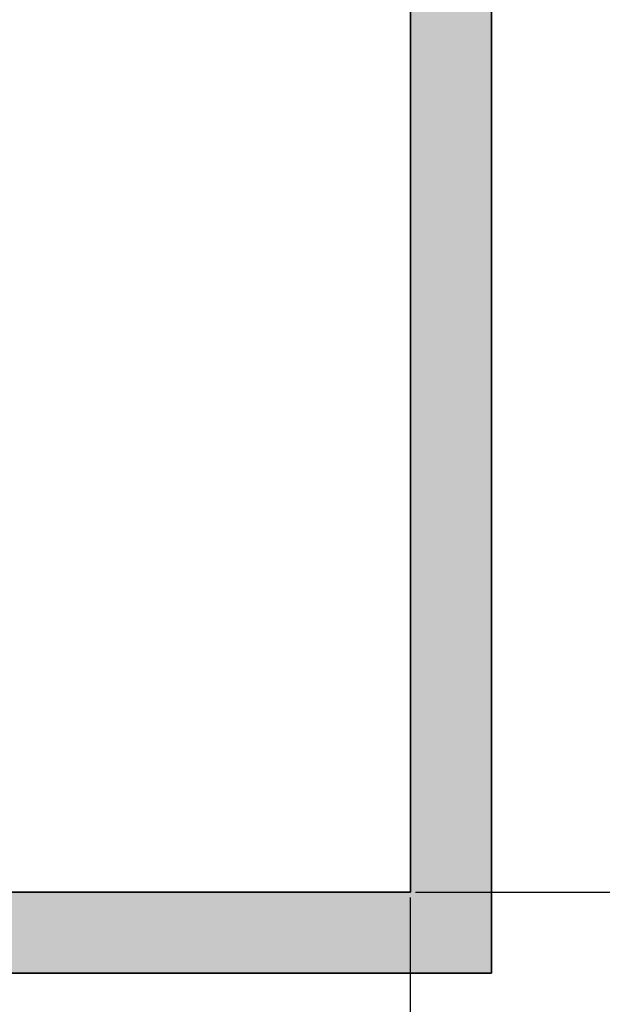
# Model space of a CAD drawing. Units: millimetres. Extents: x -22994 to 29398, y -19990 to 20176.
# Tile 36 of 135: x 183.3 to 190.48, y 29.61 to 41.76. Entities that reach past the tile are written whole.
import ezdxf
from ezdxf import colors
from ezdxf.entities.mleader import LeaderData, LeaderLine
from ezdxf.math import Vec2, Vec3

# ---------------------------------------------------------------- set-up
doc = ezdxf.new("R2010")
doc.units = ezdxf.units.MM
doc.header["$MEASUREMENT"] = 0
for name, color, linetype, lineweight in [('M-ANNO-TEXT', 7, 'Continuous', 25), ('M-DIMS', 2, 'Continuous', 18), ('M-EQPM-PATT', 7, 'Continuous', 18), ('M-PIPE', 7, 'Continuous', 35)]:
    doc.layers.add(name, color=color, linetype=linetype, lineweight=lineweight)
doc.styles.get("Standard").update_dxf_attribs({"font": 'arial.ttf'})
doc.dimstyles.get("Standard").update_dxf_attribs({"dimtxt": 0.18, "dimasz": 10000, "dimexe": 0.18, "dimexo": 0.0625, "dimgap": 0.09, "dimtad": 0, "dimtih": 1, "dimtoh": 1, "dimdec": 0, "dimzin": 0, "dimdsep": 46, "dimtxsty": 'Standard', "dimcen": 0.09, "dimadec": 0, "dimazin": 0, "dimtfac": 1, "dimtdec": 0, "dimtofl": 0, "dimtmove": 0, "dimatfit": 3, "dimfxl": 1, "dimtolj": 1, "dimtzin": 0, "dimlwd": 30, "dimarcsym": 0})

# ---------------------------------------------------------------- blocks, each defined once
blk = doc.blocks.new('*D2')
at = {"layer": 'Defpoints', "color": 0, "transparency": 16777216}
for p in [(6.677, 10.271), (290.852, 10.271), (290.852, -5.079)]:
    blk.add_point(p, dxfattribs=at)
at = {"layer": 'M-DIMS', "color": 0, "lineweight": -2, "transparency": 16777216}
for p, q in [((6.677, 10.209), (6.677, -5.259)), ((290.852, 10.209), (290.852, -5.259))]:
    blk.add_line(p, q, dxfattribs=at)
at = {"layer": 'M-DIMS', "color": 0, "lineweight": 30, "transparency": 16777216}
for p, q in [((-9993.323, -5.079), (-19993.323, -5.079)), ((10290.852, -5.079), (20290.852, -5.079))]:
    blk.add_line(p, q, dxfattribs=at)
at = {"layer": 'M-DIMS', "color": 0, "transparency": 16777216}
for points in [[(-9993.323, 1661.588), (-9993.323, -1671.745), (6.677, -5.079)], [(10290.852, 1661.588), (10290.852, -1671.745), (290.852, -5.079)]]:
    blk.add_solid(points, dxfattribs=at)
at = {"layer": 'M-DIMS', "color": 0, "transparency": 16777216, "insert": (148.765, -5.079), "char_height": 0.18, "attachment_point": 5}
blk.add_mtext('\\A1;284.2', dxfattribs=at)
blk = doc.blocks.new('*D3')
at = {"layer": 'Defpoints', "color": 0, "transparency": 16777216}
for p in [(110.265, 204.165), (110.265, 176.366), (95.833, 127.967)]:
    blk.add_point(p, dxfattribs=at)
at = {"layer": 'M-DIMS', "color": 0, "lineweight": -2, "transparency": 16777216}
for p, q in [((95.833, 128.03), (95.833, 204.345)), ((110.265, 176.429), (110.265, 204.345))]:
    blk.add_line(p, q, dxfattribs=at)
at = {"layer": 'M-DIMS', "color": 0, "lineweight": 30, "transparency": 16777216}
for p, q in [((-9904.167, 204.165), (-19904.167, 204.165)), ((10110.265, 204.165), (20110.265, 204.165))]:
    blk.add_line(p, q, dxfattribs=at)
at = {"layer": 'M-DIMS', "color": 0, "transparency": 16777216}
for points in [[(-9904.167, 1870.832), (-9904.167, -1462.501), (95.833, 204.165)], [(10110.265, 1870.832), (10110.265, -1462.501), (110.265, 204.165)]]:
    blk.add_solid(points, dxfattribs=at)
at = {"layer": 'M-DIMS', "color": 0, "transparency": 16777216, "insert": (103.049, 204.165), "char_height": 0.18, "attachment_point": 5}
blk.add_mtext('\\A1;14.432', dxfattribs=at)
blk = doc.blocks.new('*D4')
at = {"layer": 'Defpoints', "color": 0, "transparency": 16777216}
for p in [(116.265, 204.165), (110.265, 176.366), (116.265, 176.366)]:
    blk.add_point(p, dxfattribs=at)
at = {"layer": 'M-DIMS', "color": 0, "lineweight": -2, "transparency": 16777216}
for p, q in [((110.265, 176.429), (110.265, 204.345)), ((116.265, 176.429), (116.265, 204.345))]:
    blk.add_line(p, q, dxfattribs=at)
at = {"layer": 'M-DIMS', "color": 0, "lineweight": 30, "transparency": 16777216}
for p, q in [((-9889.735, 204.165), (-19889.735, 204.165)), ((10116.265, 204.165), (20116.265, 204.165))]:
    blk.add_line(p, q, dxfattribs=at)
at = {"layer": 'M-DIMS', "color": 0, "transparency": 16777216}
for points in [[(-9889.735, 1870.832), (-9889.735, -1462.501), (110.265, 204.165)], [(10116.265, 1870.832), (10116.265, -1462.501), (116.265, 204.165)]]:
    blk.add_solid(points, dxfattribs=at)
at = {"layer": 'M-DIMS', "color": 0, "transparency": 16777216, "insert": (113.265, 204.165), "char_height": 0.18, "attachment_point": 5}
blk.add_mtext('\\A1;6', dxfattribs=at)
blk = doc.blocks.new('*D5')
at = {"layer": 'Defpoints', "color": 0, "transparency": 16777216}
for p in [(181.265, 204.165), (116.265, 176.366), (181.265, 176.366)]:
    blk.add_point(p, dxfattribs=at)
at = {"layer": 'M-DIMS', "color": 0, "lineweight": -2, "transparency": 16777216}
for p, q in [((116.265, 176.429), (116.265, 204.345)), ((181.265, 176.429), (181.265, 204.345))]:
    blk.add_line(p, q, dxfattribs=at)
at = {"layer": 'M-DIMS', "color": 0, "lineweight": 30, "transparency": 16777216}
for p, q in [((-9883.735, 204.165), (-19883.735, 204.165)), ((10181.265, 204.165), (20181.265, 204.165))]:
    blk.add_line(p, q, dxfattribs=at)
at = {"layer": 'M-DIMS', "color": 0, "transparency": 16777216}
for points in [[(-9883.735, 1870.832), (-9883.735, -1462.501), (116.265, 204.165)], [(10181.265, 1870.832), (10181.265, -1462.501), (181.265, 204.165)]]:
    blk.add_solid(points, dxfattribs=at)
at = {"layer": 'M-DIMS', "color": 0, "transparency": 16777216, "insert": (148.765, 204.165), "char_height": 0.18, "attachment_point": 5}
blk.add_mtext('\\A1;65', dxfattribs=at)
blk = doc.blocks.new('*D6')
at = {"layer": 'Defpoints', "color": 0, "transparency": 16777216}
for p in [(187.265, 204.165), (181.265, 176.366), (187.265, 176.366)]:
    blk.add_point(p, dxfattribs=at)
at = {"layer": 'M-DIMS', "color": 0, "lineweight": -2, "transparency": 16777216}
for p, q in [((181.265, 176.429), (181.265, 204.345)), ((187.265, 176.429), (187.265, 204.345))]:
    blk.add_line(p, q, dxfattribs=at)
at = {"layer": 'M-DIMS', "color": 0, "lineweight": 30, "transparency": 16777216}
for p, q in [((-9818.735, 204.165), (-19818.735, 204.165)), ((10187.265, 204.165), (20187.265, 204.165))]:
    blk.add_line(p, q, dxfattribs=at)
at = {"layer": 'M-DIMS', "color": 0, "transparency": 16777216}
for points in [[(-9818.735, 1870.832), (-9818.735, -1462.501), (181.265, 204.165)], [(10187.265, 1870.832), (10187.265, -1462.501), (187.265, 204.165)]]:
    blk.add_solid(points, dxfattribs=at)
at = {"layer": 'M-DIMS', "color": 0, "transparency": 16777216, "insert": (184.265, 204.165), "char_height": 0.18, "attachment_point": 5}
blk.add_mtext('\\A1;6', dxfattribs=at)
blk = doc.blocks.new('*D7')
at = {"layer": 'Defpoints', "color": 0, "transparency": 16777216}
for p in [(201.697, 204.165), (187.265, 176.366), (201.697, 127.967)]:
    blk.add_point(p, dxfattribs=at)
at = {"layer": 'M-DIMS', "color": 0, "lineweight": -2, "transparency": 16777216}
for p, q in [((187.265, 176.429), (187.265, 204.345)), ((201.697, 128.03), (201.697, 204.345))]:
    blk.add_line(p, q, dxfattribs=at)
at = {"layer": 'M-DIMS', "color": 0, "lineweight": 30, "transparency": 16777216}
for p, q in [((-9812.735, 204.165), (-19812.735, 204.165)), ((10201.697, 204.165), (20201.697, 204.165))]:
    blk.add_line(p, q, dxfattribs=at)
at = {"layer": 'M-DIMS', "color": 0, "transparency": 16777216}
for points in [[(-9812.735, 1870.832), (-9812.735, -1462.501), (187.265, 204.165)], [(10201.697, 1870.832), (10201.697, -1462.501), (201.697, 204.165)]]:
    blk.add_solid(points, dxfattribs=at)
at = {"layer": 'M-DIMS', "color": 0, "transparency": 16777216, "insert": (194.481, 204.165), "char_height": 0.18, "attachment_point": 5}
blk.add_mtext('\\A1;14.432', dxfattribs=at)
blk = doc.blocks.new('*D8')
at = {"layer": 'Defpoints', "color": 0, "transparency": 16777216}
for p in [(227.648, 204.165), (227.648, 146.73), (201.697, 127.967)]:
    blk.add_point(p, dxfattribs=at)
at = {"layer": 'M-DIMS', "color": 0, "lineweight": -2, "transparency": 16777216}
for p, q in [((201.697, 128.03), (201.697, 204.345)), ((227.648, 146.792), (227.648, 204.345))]:
    blk.add_line(p, q, dxfattribs=at)
at = {"layer": 'M-DIMS', "color": 0, "lineweight": 30, "transparency": 16777216}
for p, q in [((-9798.303, 204.165), (-19798.303, 204.165)), ((10227.648, 204.165), (20227.648, 204.165))]:
    blk.add_line(p, q, dxfattribs=at)
at = {"layer": 'M-DIMS', "color": 0, "transparency": 16777216}
for points in [[(-9798.303, 1870.832), (-9798.303, -1462.501), (201.697, 204.165)], [(10227.648, 1870.832), (10227.648, -1462.501), (227.648, 204.165)]]:
    blk.add_solid(points, dxfattribs=at)
at = {"layer": 'M-DIMS', "color": 0, "transparency": 16777216, "insert": (214.673, 204.165), "char_height": 0.18, "attachment_point": 5}
blk.add_mtext('\\A1;25.95', dxfattribs=at)
blk = doc.blocks.new('*D9')
at = {"layer": 'Defpoints', "color": 0, "transparency": 16777216}
for p in [(187.265, 176.366), (306.202, 176.366), (290.852, 10.271)]:
    blk.add_point(p, dxfattribs=at)
at = {"layer": 'M-DIMS', "color": 0, "lineweight": 30, "transparency": 16777216}
for p, q in [((306.202, 10176.366), (306.202, 20176.366)), ((306.202, -9989.729), (306.202, -19989.729))]:
    blk.add_line(p, q, dxfattribs=at)
at = {"layer": 'M-DIMS', "color": 0, "lineweight": -2, "transparency": 16777216}
for p, q in [((187.327, 176.366), (306.382, 176.366)), ((290.915, 10.271), (306.382, 10.271))]:
    blk.add_line(p, q, dxfattribs=at)
at = {"layer": 'M-DIMS', "color": 0, "transparency": 16777216}
for points in [[(-1360.465, 10176.366), (1972.869, 10176.366), (306.202, 176.366)], [(-1360.465, -9989.729), (1972.869, -9989.729), (306.202, 10.271)]]:
    blk.add_solid(points, dxfattribs=at)
at = {"layer": 'M-DIMS', "color": 0, "transparency": 16777216, "insert": (306.202, 93.319), "char_height": 0.18, "attachment_point": 5}
blk.add_mtext('\\A1;166.1', dxfattribs=at)
blk = doc.blocks.new('*D10')
at = {"layer": 'Defpoints', "color": 0, "transparency": 16777216}
for p in [(125.65, 136.071), (133.346, 136.071), (133.346, -5.079)]:
    blk.add_point(p, dxfattribs=at)
at = {"layer": 'M-DIMS', "color": 0, "lineweight": -2, "transparency": 16777216}
for p, q in [((125.65, 136.009), (125.65, -5.259)), ((133.346, 136.009), (133.346, -5.259))]:
    blk.add_line(p, q, dxfattribs=at)
at = {"layer": 'M-DIMS', "color": 0, "lineweight": 30, "transparency": 16777216}
for p, q in [((-9874.35, -5.079), (-19874.35, -5.079)), ((10133.346, -5.079), (20133.346, -5.079))]:
    blk.add_line(p, q, dxfattribs=at)
at = {"layer": 'M-DIMS', "color": 0, "transparency": 16777216}
for points in [[(-9874.35, 1661.588), (-9874.35, -1671.745), (125.65, -5.079)], [(10133.346, 1661.588), (10133.346, -1671.745), (133.346, -5.079)]]:
    blk.add_solid(points, dxfattribs=at)
at = {"layer": 'M-DIMS', "color": 0, "transparency": 16777216, "insert": (129.498, -5.079), "char_height": 0.18, "attachment_point": 5}
blk.add_mtext('\\A1;7.696', dxfattribs=at)
blk = doc.blocks.new('*D11')
at = {"layer": 'Defpoints', "color": 0, "transparency": 16777216}
for p in [(133.346, 136.071), (135.65, 136.071), (135.65, -5.079)]:
    blk.add_point(p, dxfattribs=at)
at = {"layer": 'M-DIMS', "color": 0, "lineweight": -2, "transparency": 16777216}
for p, q in [((133.346, 136.009), (133.346, -5.259)), ((135.65, 136.009), (135.65, -5.259))]:
    blk.add_line(p, q, dxfattribs=at)
at = {"layer": 'M-DIMS', "color": 0, "lineweight": 30, "transparency": 16777216}
for p, q in [((-9866.654, -5.079), (-19866.654, -5.079)), ((10135.65, -5.079), (20135.65, -5.079))]:
    blk.add_line(p, q, dxfattribs=at)
at = {"layer": 'M-DIMS', "color": 0, "transparency": 16777216}
for points in [[(-9866.654, 1661.588), (-9866.654, -1671.745), (133.346, -5.079)], [(10135.65, 1661.588), (10135.65, -1671.745), (135.65, -5.079)]]:
    blk.add_solid(points, dxfattribs=at)
at = {"layer": 'M-DIMS', "color": 0, "transparency": 16777216, "insert": (134.498, -5.079), "char_height": 0.18, "attachment_point": 5}
blk.add_mtext('\\A1;2.304', dxfattribs=at)
blk = doc.blocks.new('*D12')
at = {"layer": 'Defpoints', "color": 0, "transparency": 16777216}
for p in [(135.65, 136.071), (145.65, 136.071), (145.65, -5.079)]:
    blk.add_point(p, dxfattribs=at)
at = {"layer": 'M-DIMS', "color": 0, "lineweight": -2, "transparency": 16777216}
for p, q in [((135.65, 136.009), (135.65, -5.259)), ((145.65, 136.009), (145.65, -5.259))]:
    blk.add_line(p, q, dxfattribs=at)
at = {"layer": 'M-DIMS', "color": 0, "lineweight": 30, "transparency": 16777216}
for p, q in [((-9864.35, -5.079), (-19864.35, -5.079)), ((10145.65, -5.079), (20145.65, -5.079))]:
    blk.add_line(p, q, dxfattribs=at)
at = {"layer": 'M-DIMS', "color": 0, "transparency": 16777216}
for points in [[(-9864.35, 1661.588), (-9864.35, -1671.745), (135.65, -5.079)], [(10145.65, 1661.588), (10145.65, -1671.745), (145.65, -5.079)]]:
    blk.add_solid(points, dxfattribs=at)
at = {"layer": 'M-DIMS', "color": 0, "transparency": 16777216, "insert": (140.65, -5.079), "char_height": 0.18, "attachment_point": 5}
blk.add_mtext('\\A1;10', dxfattribs=at)
blk = doc.blocks.new('*D13')
at = {"layer": 'Defpoints', "color": 0, "transparency": 16777216}
for p in [(145.65, 136.071), (155.65, 136.071), (155.65, -5.079)]:
    blk.add_point(p, dxfattribs=at)
at = {"layer": 'M-DIMS', "color": 0, "lineweight": -2, "transparency": 16777216}
for p, q in [((145.65, 136.009), (145.65, -5.259)), ((155.65, 136.009), (155.65, -5.259))]:
    blk.add_line(p, q, dxfattribs=at)
at = {"layer": 'M-DIMS', "color": 0, "lineweight": 30, "transparency": 16777216}
for p, q in [((-9854.35, -5.079), (-19854.35, -5.079)), ((10155.65, -5.079), (20155.65, -5.079))]:
    blk.add_line(p, q, dxfattribs=at)
at = {"layer": 'M-DIMS', "color": 0, "transparency": 16777216}
for points in [[(-9854.35, 1661.588), (-9854.35, -1671.745), (145.65, -5.079)], [(10155.65, 1661.588), (10155.65, -1671.745), (155.65, -5.079)]]:
    blk.add_solid(points, dxfattribs=at)
at = {"layer": 'M-DIMS', "color": 0, "transparency": 16777216, "insert": (150.65, -5.079), "char_height": 0.18, "attachment_point": 5}
blk.add_mtext('\\A1;10', dxfattribs=at)
blk = doc.blocks.new('*D14')
at = {"layer": 'Defpoints', "color": 0, "transparency": 16777216}
for p in [(155.65, 136.071), (165.65, 136.071), (165.65, -5.079)]:
    blk.add_point(p, dxfattribs=at)
at = {"layer": 'M-DIMS', "color": 0, "lineweight": -2, "transparency": 16777216}
for p, q in [((155.65, 136.009), (155.65, -5.259)), ((165.65, 136.009), (165.65, -5.259))]:
    blk.add_line(p, q, dxfattribs=at)
at = {"layer": 'M-DIMS', "color": 0, "lineweight": 30, "transparency": 16777216}
for p, q in [((-9844.35, -5.079), (-19844.35, -5.079)), ((10165.65, -5.079), (20165.65, -5.079))]:
    blk.add_line(p, q, dxfattribs=at)
at = {"layer": 'M-DIMS', "color": 0, "transparency": 16777216}
for points in [[(-9844.35, 1661.588), (-9844.35, -1671.745), (155.65, -5.079)], [(10165.65, 1661.588), (10165.65, -1671.745), (165.65, -5.079)]]:
    blk.add_solid(points, dxfattribs=at)
at = {"layer": 'M-DIMS', "color": 0, "transparency": 16777216, "insert": (160.65, -5.079), "char_height": 0.18, "attachment_point": 5}
blk.add_mtext('\\A1;10', dxfattribs=at)
blk = doc.blocks.new('*D15')
at = {"layer": 'Defpoints', "color": 0, "transparency": 16777216}
for p in [(173.346, 154.788), (173.346, 136.071), (306.202, 136.071)]:
    blk.add_point(p, dxfattribs=at)
at = {"layer": 'M-DIMS', "color": 0, "lineweight": 30, "transparency": 16777216}
for p, q in [((306.202, 10154.788), (306.202, 20154.788)), ((306.202, -9863.929), (306.202, -19863.929))]:
    blk.add_line(p, q, dxfattribs=at)
at = {"layer": 'M-DIMS', "color": 0, "lineweight": -2, "transparency": 16777216}
for p, q in [((173.408, 154.788), (306.382, 154.788)), ((173.408, 136.071), (306.382, 136.071))]:
    blk.add_line(p, q, dxfattribs=at)
at = {"layer": 'M-DIMS', "color": 0, "transparency": 16777216}
for points in [[(-1360.465, 10154.788), (1972.869, 10154.788), (306.202, 154.788)], [(-1360.465, -9863.929), (1972.869, -9863.929), (306.202, 136.071)]]:
    blk.add_solid(points, dxfattribs=at)
at = {"layer": 'M-DIMS', "color": 0, "transparency": 16777216, "insert": (306.202, 145.43), "char_height": 0.18, "attachment_point": 5}
blk.add_mtext('\\A1;18.717', dxfattribs=at)
blk = doc.blocks.new('*D16')
at = {"layer": 'Defpoints', "color": 0, "transparency": 16777216}
for p in [(120.17, 204.165), (110.466, 48.035), (120.17, 48.035)]:
    blk.add_point(p, dxfattribs=at)
at = {"layer": 'M-DIMS', "color": 0, "lineweight": -2, "transparency": 16777216}
for p, q in [((110.466, 48.097), (110.466, 204.345)), ((120.17, 48.097), (120.17, 204.345))]:
    blk.add_line(p, q, dxfattribs=at)
at = {"layer": 'M-DIMS', "color": 0, "lineweight": 30, "transparency": 16777216}
for p, q in [((-9889.534, 204.165), (-19889.534, 204.165)), ((10120.17, 204.165), (20120.17, 204.165))]:
    blk.add_line(p, q, dxfattribs=at)
at = {"layer": 'M-DIMS', "color": 0, "transparency": 16777216}
for points in [[(-9889.534, 1870.832), (-9889.534, -1462.501), (110.466, 204.165)], [(10120.17, 1870.832), (10120.17, -1462.501), (120.17, 204.165)]]:
    blk.add_solid(points, dxfattribs=at)
at = {"layer": 'M-DIMS', "color": 0, "transparency": 16777216, "insert": (115.318, 204.165), "char_height": 0.18, "attachment_point": 5}
blk.add_mtext('\\A1;9.704', dxfattribs=at)
blk = doc.blocks.new('*D17')
at = {"layer": 'Defpoints', "color": 0, "transparency": 16777216}
for p in [(126.17, 204.165), (120.17, 48.035), (126.17, 48.035)]:
    blk.add_point(p, dxfattribs=at)
at = {"layer": 'M-DIMS', "color": 0, "lineweight": -2, "transparency": 16777216}
for p, q in [((120.17, 48.097), (120.17, 204.345)), ((126.17, 48.097), (126.17, 204.345))]:
    blk.add_line(p, q, dxfattribs=at)
at = {"layer": 'M-DIMS', "color": 0, "lineweight": 30, "transparency": 16777216}
for p, q in [((-9879.83, 204.165), (-19879.83, 204.165)), ((10126.17, 204.165), (20126.17, 204.165))]:
    blk.add_line(p, q, dxfattribs=at)
at = {"layer": 'M-DIMS', "color": 0, "transparency": 16777216}
for points in [[(-9879.83, 1870.832), (-9879.83, -1462.501), (120.17, 204.165)], [(10126.17, 1870.832), (10126.17, -1462.501), (126.17, 204.165)]]:
    blk.add_solid(points, dxfattribs=at)
at = {"layer": 'M-DIMS', "color": 0, "transparency": 16777216, "insert": (123.17, 204.165), "char_height": 0.18, "attachment_point": 5}
blk.add_mtext('\\A1;6', dxfattribs=at)
blk = doc.blocks.new('*D18')
at = {"layer": 'Defpoints', "color": 0, "transparency": 16777216}
for p in [(132.17, 204.165), (126.17, 48.035), (132.17, 48.035)]:
    blk.add_point(p, dxfattribs=at)
at = {"layer": 'M-DIMS', "color": 0, "lineweight": -2, "transparency": 16777216}
for p, q in [((126.17, 48.097), (126.17, 204.345)), ((132.17, 48.097), (132.17, 204.345))]:
    blk.add_line(p, q, dxfattribs=at)
at = {"layer": 'M-DIMS', "color": 0, "lineweight": 30, "transparency": 16777216}
for p, q in [((-9873.83, 204.165), (-19873.83, 204.165)), ((10132.17, 204.165), (20132.17, 204.165))]:
    blk.add_line(p, q, dxfattribs=at)
at = {"layer": 'M-DIMS', "color": 0, "transparency": 16777216}
for points in [[(-9873.83, 1870.832), (-9873.83, -1462.501), (126.17, 204.165)], [(10132.17, 1870.832), (10132.17, -1462.501), (132.17, 204.165)]]:
    blk.add_solid(points, dxfattribs=at)
at = {"layer": 'M-DIMS', "color": 0, "transparency": 16777216, "insert": (129.17, 204.165), "char_height": 0.18, "attachment_point": 5}
blk.add_mtext('\\A1;6', dxfattribs=at)
blk = doc.blocks.new('*D19')
at = {"layer": 'Defpoints', "color": 0, "transparency": 16777216}
for p in [(138.17, 204.165), (132.17, 48.035), (138.17, 48.035)]:
    blk.add_point(p, dxfattribs=at)
at = {"layer": 'M-DIMS', "color": 0, "lineweight": -2, "transparency": 16777216}
for p, q in [((132.17, 48.097), (132.17, 204.345)), ((138.17, 48.097), (138.17, 204.345))]:
    blk.add_line(p, q, dxfattribs=at)
at = {"layer": 'M-DIMS', "color": 0, "lineweight": 30, "transparency": 16777216}
for p, q in [((-9867.83, 204.165), (-19867.83, 204.165)), ((10138.17, 204.165), (20138.17, 204.165))]:
    blk.add_line(p, q, dxfattribs=at)
at = {"layer": 'M-DIMS', "color": 0, "transparency": 16777216}
for points in [[(-9867.83, 1870.832), (-9867.83, -1462.501), (132.17, 204.165)], [(10138.17, 1870.832), (10138.17, -1462.501), (138.17, 204.165)]]:
    blk.add_solid(points, dxfattribs=at)
at = {"layer": 'M-DIMS', "color": 0, "transparency": 16777216, "insert": (135.17, 204.165), "char_height": 0.18, "attachment_point": 5}
blk.add_mtext('\\A1;6', dxfattribs=at)
blk = doc.blocks.new('*D20')
at = {"layer": 'Defpoints', "color": 0, "transparency": 16777216}
for p in [(144.17, 204.165), (138.17, 48.035), (144.17, 48.035)]:
    blk.add_point(p, dxfattribs=at)
at = {"layer": 'M-DIMS', "color": 0, "lineweight": -2, "transparency": 16777216}
for p, q in [((138.17, 48.097), (138.17, 204.345)), ((144.17, 48.097), (144.17, 204.345))]:
    blk.add_line(p, q, dxfattribs=at)
at = {"layer": 'M-DIMS', "color": 0, "lineweight": 30, "transparency": 16777216}
for p, q in [((-9861.83, 204.165), (-19861.83, 204.165)), ((10144.17, 204.165), (20144.17, 204.165))]:
    blk.add_line(p, q, dxfattribs=at)
at = {"layer": 'M-DIMS', "color": 0, "transparency": 16777216}
for points in [[(-9861.83, 1870.832), (-9861.83, -1462.501), (138.17, 204.165)], [(10144.17, 1870.832), (10144.17, -1462.501), (144.17, 204.165)]]:
    blk.add_solid(points, dxfattribs=at)
at = {"layer": 'M-DIMS', "color": 0, "transparency": 16777216, "insert": (141.17, 204.165), "char_height": 0.18, "attachment_point": 5}
blk.add_mtext('\\A1;6', dxfattribs=at)
blk = doc.blocks.new('*D21')
at = {"layer": 'Defpoints', "color": 0, "transparency": 16777216}
for p in [(149.116, 204.165), (144.17, 48.035), (149.116, 48.035)]:
    blk.add_point(p, dxfattribs=at)
at = {"layer": 'M-DIMS', "color": 0, "lineweight": -2, "transparency": 16777216}
for p, q in [((144.17, 48.097), (144.17, 204.345)), ((149.116, 48.097), (149.116, 204.345))]:
    blk.add_line(p, q, dxfattribs=at)
at = {"layer": 'M-DIMS', "color": 0, "lineweight": 30, "transparency": 16777216}
for p, q in [((-9855.83, 204.165), (-19855.83, 204.165)), ((10149.116, 204.165), (20149.116, 204.165))]:
    blk.add_line(p, q, dxfattribs=at)
at = {"layer": 'M-DIMS', "color": 0, "transparency": 16777216}
for points in [[(-9855.83, 1870.832), (-9855.83, -1462.501), (144.17, 204.165)], [(10149.116, 1870.832), (10149.116, -1462.501), (149.116, 204.165)]]:
    blk.add_solid(points, dxfattribs=at)
at = {"layer": 'M-DIMS', "color": 0, "transparency": 16777216, "insert": (146.643, 204.165), "char_height": 0.18, "attachment_point": 5}
blk.add_mtext('\\A1;4.945', dxfattribs=at)
blk = doc.blocks.new('*D22')
at = {"layer": 'Defpoints', "color": 0, "transparency": 16777216}
for p in [(149.116, 30.99), (155.116, 30.99), (155.116, -5.079)]:
    blk.add_point(p, dxfattribs=at)
at = {"layer": 'M-DIMS', "color": 0, "lineweight": -2, "transparency": 16777216}
for p, q in [((149.116, 30.927), (149.116, -5.259)), ((155.116, 30.927), (155.116, -5.259))]:
    blk.add_line(p, q, dxfattribs=at)
at = {"layer": 'M-DIMS', "color": 0, "lineweight": 30, "transparency": 16777216}
for p, q in [((-9850.884, -5.079), (-19850.884, -5.079)), ((10155.116, -5.079), (20155.116, -5.079))]:
    blk.add_line(p, q, dxfattribs=at)
at = {"layer": 'M-DIMS', "color": 0, "transparency": 16777216}
for points in [[(-9850.884, 1661.588), (-9850.884, -1671.745), (149.116, -5.079)], [(10155.116, 1661.588), (10155.116, -1671.745), (155.116, -5.079)]]:
    blk.add_solid(points, dxfattribs=at)
at = {"layer": 'M-DIMS', "color": 0, "transparency": 16777216, "insert": (152.116, -5.079), "char_height": 0.18, "attachment_point": 5}
blk.add_mtext('\\A1;6', dxfattribs=at)
blk = doc.blocks.new('*D23')
at = {"layer": 'Defpoints', "color": 0, "transparency": 16777216}
for p in [(155.116, 30.99), (161.116, 30.99), (161.116, -5.079)]:
    blk.add_point(p, dxfattribs=at)
at = {"layer": 'M-DIMS', "color": 0, "lineweight": -2, "transparency": 16777216}
for p, q in [((155.116, 30.927), (155.116, -5.259)), ((161.116, 30.927), (161.116, -5.259))]:
    blk.add_line(p, q, dxfattribs=at)
at = {"layer": 'M-DIMS', "color": 0, "lineweight": 30, "transparency": 16777216}
for p, q in [((-9844.884, -5.079), (-19844.884, -5.079)), ((10161.116, -5.079), (20161.116, -5.079))]:
    blk.add_line(p, q, dxfattribs=at)
at = {"layer": 'M-DIMS', "color": 0, "transparency": 16777216}
for points in [[(-9844.884, 1661.588), (-9844.884, -1671.745), (155.116, -5.079)], [(10161.116, 1661.588), (10161.116, -1671.745), (161.116, -5.079)]]:
    blk.add_solid(points, dxfattribs=at)
at = {"layer": 'M-DIMS', "color": 0, "transparency": 16777216, "insert": (158.116, -5.079), "char_height": 0.18, "attachment_point": 5}
blk.add_mtext('\\A1;6', dxfattribs=at)
blk = doc.blocks.new('*D24')
at = {"layer": 'Defpoints', "color": 0, "transparency": 16777216}
for p in [(161.116, 30.99), (166.439, 30.99), (166.439, -5.079)]:
    blk.add_point(p, dxfattribs=at)
at = {"layer": 'M-DIMS', "color": 0, "lineweight": -2, "transparency": 16777216}
for p, q in [((161.116, 30.927), (161.116, -5.259)), ((166.439, 30.927), (166.439, -5.259))]:
    blk.add_line(p, q, dxfattribs=at)
at = {"layer": 'M-DIMS', "color": 0, "lineweight": 30, "transparency": 16777216}
for p, q in [((-9838.884, -5.079), (-19838.884, -5.079)), ((10166.439, -5.079), (20166.439, -5.079))]:
    blk.add_line(p, q, dxfattribs=at)
at = {"layer": 'M-DIMS', "color": 0, "transparency": 16777216}
for points in [[(-9838.884, 1661.588), (-9838.884, -1671.745), (161.116, -5.079)], [(10166.439, 1661.588), (10166.439, -1671.745), (166.439, -5.079)]]:
    blk.add_solid(points, dxfattribs=at)
at = {"layer": 'M-DIMS', "color": 0, "transparency": 16777216, "insert": (163.777, -5.079), "char_height": 0.18, "attachment_point": 5}
blk.add_mtext('\\A1;5.323', dxfattribs=at)
blk = doc.blocks.new('*D25')
at = {"layer": 'Defpoints', "color": 0, "transparency": 16777216}
for p in [(166.439, 30.99), (172.439, 30.99), (172.439, -5.079)]:
    blk.add_point(p, dxfattribs=at)
at = {"layer": 'M-DIMS', "color": 0, "lineweight": -2, "transparency": 16777216}
for p, q in [((166.439, 30.927), (166.439, -5.259)), ((172.439, 30.927), (172.439, -5.259))]:
    blk.add_line(p, q, dxfattribs=at)
at = {"layer": 'M-DIMS', "color": 0, "lineweight": 30, "transparency": 16777216}
for p, q in [((-9833.561, -5.079), (-19833.561, -5.079)), ((10172.439, -5.079), (20172.439, -5.079))]:
    blk.add_line(p, q, dxfattribs=at)
at = {"layer": 'M-DIMS', "color": 0, "transparency": 16777216}
for points in [[(-9833.561, 1661.588), (-9833.561, -1671.745), (166.439, -5.079)], [(10172.439, 1661.588), (10172.439, -1671.745), (172.439, -5.079)]]:
    blk.add_solid(points, dxfattribs=at)
at = {"layer": 'M-DIMS', "color": 0, "transparency": 16777216, "insert": (169.439, -5.079), "char_height": 0.18, "attachment_point": 5}
blk.add_mtext('\\A1;6', dxfattribs=at)
blk = doc.blocks.new('*D26')
at = {"layer": 'Defpoints', "color": 0, "transparency": 16777216}
for p in [(172.439, 30.99), (178.439, 30.99), (178.439, -5.079)]:
    blk.add_point(p, dxfattribs=at)
at = {"layer": 'M-DIMS', "color": 0, "lineweight": -2, "transparency": 16777216}
for p, q in [((172.439, 30.927), (172.439, -5.259)), ((178.439, 30.927), (178.439, -5.259))]:
    blk.add_line(p, q, dxfattribs=at)
at = {"layer": 'M-DIMS', "color": 0, "lineweight": 30, "transparency": 16777216}
for p, q in [((-9827.561, -5.079), (-19827.561, -5.079)), ((10178.439, -5.079), (20178.439, -5.079))]:
    blk.add_line(p, q, dxfattribs=at)
at = {"layer": 'M-DIMS', "color": 0, "transparency": 16777216}
for points in [[(-9827.561, 1661.588), (-9827.561, -1671.745), (172.439, -5.079)], [(10178.439, 1661.588), (10178.439, -1671.745), (178.439, -5.079)]]:
    blk.add_solid(points, dxfattribs=at)
at = {"layer": 'M-DIMS', "color": 0, "transparency": 16777216, "insert": (175.439, -5.079), "char_height": 0.18, "attachment_point": 5}
blk.add_mtext('\\A1;6', dxfattribs=at)
blk = doc.blocks.new('*D27')
at = {"layer": 'Defpoints', "color": 0, "transparency": 16777216}
for p in [(178.439, 30.99), (188.117, 30.99), (188.117, -5.079)]:
    blk.add_point(p, dxfattribs=at)
at = {"layer": 'M-DIMS', "color": 0, "lineweight": -2, "transparency": 16777216}
for p, q in [((178.439, 30.927), (178.439, -5.259)), ((188.117, 30.927), (188.117, -5.259))]:
    blk.add_line(p, q, dxfattribs=at)
at = {"layer": 'M-DIMS', "color": 0, "lineweight": 30, "transparency": 16777216}
for p, q in [((-9821.561, -5.079), (-19821.561, -5.079)), ((10188.117, -5.079), (20188.117, -5.079))]:
    blk.add_line(p, q, dxfattribs=at)
at = {"layer": 'M-DIMS', "color": 0, "transparency": 16777216}
for points in [[(-9821.561, 1661.588), (-9821.561, -1671.745), (178.439, -5.079)], [(10188.117, 1661.588), (10188.117, -1671.745), (188.117, -5.079)]]:
    blk.add_solid(points, dxfattribs=at)
at = {"layer": 'M-DIMS', "color": 0, "transparency": 16777216, "insert": (183.278, -5.079), "char_height": 0.18, "attachment_point": 5}
blk.add_mtext('\\A1;9.679', dxfattribs=at)
blk = doc.blocks.new('*D28')
at = {"layer": 'Defpoints', "color": 0, "transparency": 16777216}
for p in [(188.117, 48.035), (306.202, 48.035), (188.117, 30.99)]:
    blk.add_point(p, dxfattribs=at)
at = {"layer": 'M-DIMS', "color": 0, "lineweight": 30, "transparency": 16777216}
for p, q in [((306.202, 10048.035), (306.202, 20048.035)), ((306.202, -9969.01), (306.202, -19969.01))]:
    blk.add_line(p, q, dxfattribs=at)
at = {"layer": 'M-DIMS', "color": 0, "lineweight": -2, "transparency": 16777216}
for p, q in [((188.18, 48.035), (306.382, 48.035)), ((188.18, 30.99), (306.382, 30.99))]:
    blk.add_line(p, q, dxfattribs=at)
at = {"layer": 'M-DIMS', "color": 0, "transparency": 16777216}
for points in [[(-1360.465, 10048.035), (1972.869, 10048.035), (306.202, 48.035)], [(-1360.465, -9969.01), (1972.869, -9969.01), (306.202, 30.99)]]:
    blk.add_solid(points, dxfattribs=at)
at = {"layer": 'M-DIMS', "color": 0, "transparency": 16777216, "insert": (306.202, 39.512), "char_height": 0.18, "attachment_point": 5}
blk.add_mtext('\\A1;17.045', dxfattribs=at)
blk = doc.blocks.new('*D29')
at = {"layer": 'Defpoints', "color": 0, "transparency": 16777216}
for p in [(36.801, 80.045), (64.03, 80.045)]:
    blk.add_point(p, dxfattribs=at)
at = {"layer": 'M-DIMS', "color": 0, "lineweight": -2, "transparency": 16777216}
for p, q in [((50.415, 79.955), (50.415, 80.135)), ((50.325, 80.045), (50.505, 80.045))]:
    blk.add_line(p, q, dxfattribs=at)
at = {"layer": 'M-DIMS', "color": 0, "lineweight": 30, "transparency": 16777216}
blk.add_line((20064.03, 80.03), (10064.03, 80.038), dxfattribs=at)
at = {"layer": 'M-DIMS', "color": 0, "transparency": 16777216}
blk.add_solid([(10064.031, 1746.704), (10064.028, -1586.629), (64.03, 80.045)], dxfattribs=at)
at = {"layer": 'M-DIMS', "color": 0, "transparency": 16777216, "insert": (20064.521, 80.03), "char_height": 0.18, "attachment_point": 5}
blk.add_mtext('\\A1;∅27.23', dxfattribs=at)
blk = doc.blocks.new('*D36')
at = {"layer": 'Defpoints', "color": 0, "transparency": 16777216}
for p in [(46.39, 31.303), (46.387, 26.593)]:
    blk.add_point(p, dxfattribs=at)
at = {"layer": 'M-DIMS', "color": 0, "lineweight": 30, "transparency": 16777216}
for p, q in [((57.15, 20031.301), (51.77, 10031.302)), ((10057.15, 20031.301), (57.15, 20031.301))]:
    blk.add_line(p, q, dxfattribs=at)
at = {"layer": 'M-DIMS', "color": 0, "lineweight": -2, "transparency": 16777216}
for p, q in [((46.389, 28.858), (46.389, 29.038)), ((46.299, 28.948), (46.479, 28.948))]:
    blk.add_line(p, q, dxfattribs=at)
at = {"layer": 'M-DIMS', "color": 0, "transparency": 16777216}
blk.add_solid([(-1614.896, 10032.199), (1718.436, 10030.405), (46.39, 31.303)], dxfattribs=at)
at = {"layer": 'M-DIMS', "color": 0, "transparency": 16777216, "insert": (10057.554, 20031.301), "char_height": 0.18, "attachment_point": 5}
blk.add_mtext('\\A1;∅4.71', dxfattribs=at)
blk = doc.blocks.new('*D37')
at = {"layer": 'Defpoints', "color": 0, "transparency": 16777216}
for p in [(54.834, 118.615), (59.494, 118.614)]:
    blk.add_point(p, dxfattribs=at)
at = {"layer": 'M-DIMS', "color": 0, "lineweight": -2, "transparency": 16777216}
for p, q in [((57.164, 118.524), (57.164, 118.704)), ((57.074, 118.614), (57.254, 118.614))]:
    blk.add_line(p, q, dxfattribs=at)
at = {"layer": 'M-DIMS', "color": 0, "lineweight": 30, "transparency": 16777216}
blk.add_line((20059.493, 116.253), (10059.494, 117.434), dxfattribs=at)
at = {"layer": 'M-DIMS', "color": 0, "transparency": 16777216}
blk.add_solid([(10059.69, 1784.1), (10059.297, -1549.233), (59.494, 118.614)], dxfattribs=at)
at = {"layer": 'M-DIMS', "color": 0, "transparency": 16777216, "insert": (20059.985, 116.253), "char_height": 0.18, "attachment_point": 5}
blk.add_mtext('\\A1;∅4.659', dxfattribs=at)

msp = doc.modelspace()

# ---------------------------------------------------------------- hatches: boundary and pattern name
at = {"layer": 'M-EQPM-PATT'}
h = msp.add_hatch(color=256, dxfattribs=at)
h.set_gradient(color1=(19, 155, 72), color2=(88, 186, 72), tint=1, name='CYLINDER')
h.paths.add_polyline_path([(109.4658, 29.9895), (189.1175, 29.9895), (189.1175, 77.6953), (128.1172, 77.6953, 0.4142136), (126.1172, 75.6953), (126.1172, 73.6953, 0.4142136), (128.1172, 71.6953), (178.5136, 71.6953, -0.4142136), (179.5136, 70.6953), (179.5136, 68.6953, -0.4142136), (178.5136, 67.6953), (128.1172, 67.6953, 0.4142136), (126.1172, 65.6953), (126.1172, 63.6953, 0.4142136), (128.1172, 61.6953), (178.5136, 61.6953, -0.4142136), (179.5136, 60.6953), (179.5136, 58.6953, -0.4142136), (178.5136, 57.6953), (109.7466, 57.6953, -0.4142136), (108.7466, 58.6953), (108.7466, 75.5922, 0.4142136), (106.7466, 77.5922), (101.8327, 77.5922), (101.8327, 76.5922), (106.7466, 76.5922, -0.4142136), (107.7466, 75.5922), (107.7466, 58.6953, 0.4142136), (109.7466, 56.6953), (178.5136, 56.6953, 0.4142136), (180.5136, 58.6953), (180.5136, 60.6953, 0.4142136), (178.5136, 62.6953), (128.1172, 62.6953, -0.4142136), (127.1172, 63.6953), (127.1172, 65.6953, -0.4142136), (128.1172, 66.6953), (178.5136, 66.6953, 0.4142136), (180.5136, 68.6953), (180.5136, 70.6953, 0.4142136), (178.5136, 72.6953), (128.1172, 72.6953, -0.4142136), (127.1172, 73.6953), (127.1172, 75.6953, -0.4142136), (128.1172, 76.6953), (188.1175, 76.6953), (188.1175, 49.0349), (110.4658, 49.0349), (110.4658, 51.9576), (101.8327, 51.9576), (101.8327, 50.9576), (109.4658, 50.9576), (109.4658, 48.5349)])
h.paths.add_polyline_path([(110.4658, 48.0349), (188.1175, 48.0349), (188.1175, 30.9895), (110.4658, 30.9895)], flags=16)
h.paths.add_polyline_path([(136.1519, 78.0082), (161.2406, 78.0082), (161.2406, 84.1903), (136.1519, 84.1903)], flags=9)

# ---------------------------------------------------------------- linework, layer by layer
at = {"layer": 'M-PIPE'}
msp.add_lwpolyline([(189.1175, 29.9895), (189.1175, 77.6953), (128.1172, 77.6953, 0.4142136), (126.1172, 75.6953), (126.1172, 73.6953, 0.4142136), (128.1172, 71.6953), (178.5136, 71.6953, -0.4142136), (179.5136, 70.6953), (179.5136, 68.6953, -0.4142136), (178.5136, 67.6953), (128.1172, 67.6953, 0.4142136), (126.1172, 65.6953), (126.1172, 63.6953, 0.4142136), (128.1172, 61.6953), (178.5136, 61.6953, -0.4142136), (179.5136, 60.6953), (179.5136, 58.6953, -0.4142136), (178.5136, 57.6953), (109.7466, 57.6953, -0.4142136), (108.7466, 58.6953), (108.7466, 75.5922, 0.4142136), (106.7466, 77.5922), (101.8327, 77.5922)], format="xyb", dxfattribs=at)
for points in [[(189.1175, 29.9895), (109.4658, 29.9895), (109.4658, 49.0349)], [(188.1175, 30.9895), (110.4658, 30.9895), (110.4658, 48.0349), (188.1175, 48.0349)], [(188.1175, 30.9895), (188.1175, 48.0349)]]:
    msp.add_lwpolyline(points, dxfattribs=at)

# ---------------------------------------------------------------- dimensions: what is measured, and where the dimension line sits
at = {"layer": 'M-DIMS'}
for base, p1, p2, override, picture, middle in [((306.202, 176.3662), (290.852, 10.2713), (187.2647, 176.3662), {"dimdec": 1, "dimlfac": 1, "dimrnd": 0, "dimzin": 0, "dimdsep": 46, "dimlunit": 2}, '*D9', (306.202, 93.3187)), ((306.202, 136.0713), (173.3459, 154.788), (173.3459, 136.0713), {"dimdec": 3, "dimlfac": 1, "dimrnd": 0, "dimzin": 0, "dimdsep": 46, "dimlunit": 2}, '*D15', (306.202, 145.4297)), ((306.202, 48.0349), (188.1175, 30.9895), (188.1175, 48.0349), {"dimdec": 3, "dimlfac": 1, "dimrnd": 0, "dimzin": 0, "dimdsep": 46, "dimlunit": 2}, '*D28', (306.202, 39.5122))]:
    dim = msp.add_linear_dim(base=base, p1=p1, p2=p2, angle=90, dimstyle='Standard', override=override, dxfattribs=at)
    dim.commit()
    dim.dimension.update_dxf_attribs({"geometry": picture, "text_midpoint": middle})
dim = msp.add_diameter_dim_2p(p1=(46.3875, 26.5934), p2=(46.39, 31.3035), dimstyle='Standard', override={"dimdec": 2, "dimlfac": 1, "dimrnd": 0, "dimzin": 0, "dimdsep": 46, "dimlunit": 2}, dxfattribs=at)
dim.commit()
dim.dimension.update_dxf_attribs({"geometry": '*D36', "text_midpoint": (10057.5542, 20031.3006), "dimtype": 163})
for base, p1, p2, override, picture, middle in [((110.2647, 204.1654), (95.8327, 127.967), (110.2647, 176.3662), {"dimdec": 3, "dimlfac": 1, "dimrnd": 0, "dimzin": 0, "dimdsep": 46, "dimlunit": 2}, '*D3', (103.0487, 204.1654)), ((116.2647, 204.1654), (110.2647, 176.3662), (116.2647, 176.3662), {"dimdec": 0, "dimlfac": 1, "dimrnd": 0, "dimzin": 0, "dimdsep": 46, "dimlunit": 2}, '*D4', (113.2647, 204.1654)), ((120.1702, 204.1654), (110.4658, 48.0349), (120.1702, 48.0349), {"dimdec": 3, "dimlfac": 1, "dimrnd": 0, "dimzin": 0, "dimdsep": 46, "dimlunit": 2}, '*D16', (115.318, 204.1654)), ((181.2647, 204.1654), (116.2647, 176.3662), (181.2647, 176.3662), {"dimdec": 0, "dimlfac": 1, "dimrnd": 0, "dimzin": 0, "dimdsep": 46, "dimlunit": 2}, '*D5', (148.7647, 204.1654)), ((126.1702, 204.1654), (120.1702, 48.0349), (126.1702, 48.0349), {"dimdec": 0, "dimlfac": 1, "dimrnd": 0, "dimzin": 0, "dimdsep": 46, "dimlunit": 2}, '*D17', (123.1702, 204.1654)), ((132.1702, 204.1654), (126.1702, 48.0349), (132.1702, 48.0349), {"dimdec": 0, "dimlfac": 1, "dimrnd": 0, "dimzin": 0, "dimdsep": 46, "dimlunit": 2}, '*D18', (129.1702, 204.1654)), ((138.1702, 204.1654), (132.1702, 48.0349), (138.1702, 48.0349), {"dimdec": 0, "dimlfac": 1, "dimrnd": 0, "dimzin": 0, "dimdsep": 46, "dimlunit": 2}, '*D19', (135.1702, 204.1654)), ((144.1702, 204.1654), (138.1702, 48.0349), (144.1702, 48.0349), {"dimdec": 0, "dimlfac": 1, "dimrnd": 0, "dimzin": 0, "dimdsep": 46, "dimlunit": 2}, '*D20', (141.1702, 204.1654)), ((149.11567, 204.16539), (144.17023, 48.03494), (149.11567, 48.03494), {"dimdec": 3, "dimlfac": 1, "dimrnd": 0, "dimzin": 0, "dimdsep": 46, "dimlunit": 2}, '*D21', (146.64295, 204.16539)), ((187.2647, 204.1654), (181.2647, 176.3662), (187.2647, 176.3662), {"dimdec": 0, "dimlfac": 1, "dimrnd": 0, "dimzin": 0, "dimdsep": 46, "dimlunit": 2}, '*D6', (184.2647, 204.1654)), ((201.6967, 204.1654), (187.2647, 176.3662), (201.6967, 127.967), {"dimdec": 3, "dimlfac": 1, "dimrnd": 0, "dimzin": 0, "dimdsep": 46, "dimlunit": 2}, '*D7', (194.4807, 204.1654)), ((227.6485, 204.1654), (201.6967, 127.967), (227.6485, 146.7296), {"dimdec": 2, "dimlfac": 1, "dimrnd": 0, "dimzin": 0, "dimdsep": 46, "dimlunit": 2}, '*D8', (214.6726, 204.1654)), ((290.852, -5.0787), (6.6773, 10.2713), (290.852, 10.2713), {"dimdec": 1, "dimlfac": 1, "dimrnd": 0, "dimzin": 0, "dimdsep": 46, "dimlunit": 2}, '*D2', (148.7647, -5.0787)), ((133.3459, -5.0787), (125.6498, 136.0713), (133.3459, 136.0713), {"dimdec": 3, "dimlfac": 1, "dimrnd": 0, "dimzin": 0, "dimdsep": 46, "dimlunit": 2}, '*D10', (129.4978, -5.0787)), ((135.6498, -5.0787), (133.3459, 136.0713), (135.6498, 136.0713), {"dimdec": 3, "dimlfac": 1, "dimrnd": 0, "dimzin": 0, "dimdsep": 46, "dimlunit": 2}, '*D11', (134.4978, -5.0787)), ((145.6498, -5.0787), (135.6498, 136.0713), (145.6498, 136.0713), {"dimdec": 0, "dimlfac": 1, "dimrnd": 0, "dimzin": 0, "dimdsep": 46, "dimlunit": 2}, '*D12', (140.6498, -5.0787)), ((155.6498, -5.0787), (145.6498, 136.0713), (155.6498, 136.0713), {"dimdec": 0, "dimlfac": 1, "dimrnd": 0, "dimzin": 0, "dimdsep": 46, "dimlunit": 2}, '*D13', (150.6498, -5.0787)), ((155.1157, -5.0787), (149.1157, 30.9895), (155.1157, 30.9895), {"dimdec": 0, "dimlfac": 1, "dimrnd": 0, "dimzin": 0, "dimdsep": 46, "dimlunit": 2}, '*D22', (152.1157, -5.0787)), ((161.1157, -5.0787), (155.1157, 30.9895), (161.1157, 30.9895), {"dimdec": 0, "dimlfac": 1, "dimrnd": 0, "dimzin": 0, "dimdsep": 46, "dimlunit": 2}, '*D23', (158.1157, -5.0787)), ((165.6498, -5.0787), (155.6498, 136.0713), (165.6498, 136.0713), {"dimdec": 0, "dimlfac": 1, "dimrnd": 0, "dimzin": 0, "dimdsep": 46, "dimlunit": 2}, '*D14', (160.6498, -5.0787)), ((166.4387, -5.0787), (161.1157, 30.9895), (166.4387, 30.9895), {"dimdec": 3, "dimlfac": 1, "dimrnd": 0, "dimzin": 0, "dimdsep": 46, "dimlunit": 2}, '*D24', (163.7772, -5.0787)), ((172.4387, -5.0787), (166.4387, 30.9895), (172.4387, 30.9895), {"dimdec": 0, "dimlfac": 1, "dimrnd": 0, "dimzin": 0, "dimdsep": 46, "dimlunit": 2}, '*D25', (169.4387, -5.0787)), ((178.4387, -5.0787), (172.4387, 30.9895), (178.4387, 30.9895), {"dimdec": 0, "dimlfac": 1, "dimrnd": 0, "dimzin": 0, "dimdsep": 46, "dimlunit": 2}, '*D26', (175.4387, -5.0787)), ((188.1175, -5.0787), (178.4387, 30.9895), (188.1175, 30.9895), {"dimdec": 3, "dimlfac": 1, "dimrnd": 0, "dimzin": 0, "dimdsep": 46, "dimlunit": 2}, '*D27', (183.2781, -5.0787))]:
    dim = msp.add_linear_dim(base=base, p1=p1, p2=p2, dimstyle='Standard', override=override, dxfattribs=at)
    dim.commit()
    dim.dimension.update_dxf_attribs({"geometry": picture, "text_midpoint": middle})
for p1, p2, override, picture, middle in [((54.8343, 118.6145), (59.4936, 118.614), {"dimdec": 3, "dimlfac": 1, "dimrnd": 0, "dimzin": 0, "dimdsep": 46, "dimlunit": 2}, '*D37', (20059.4934, 116.2531)), ((36.8006, 80.045), (64.0296, 80.045), {"dimdec": 2, "dimlfac": 1, "dimrnd": 0, "dimzin": 0, "dimdsep": 46, "dimlunit": 2}, '*D29', (20064.0296, 80.0303))]:
    dim = msp.add_diameter_dim_2p(p1=p1, p2=p2, dimstyle='Standard', override=override, dxfattribs=at)
    dim.commit()
    dim.dimension.update_dxf_attribs({"geometry": picture, "text_midpoint": middle})

# ---------------------------------------------------------------- leaders
at = {"layer": 'M-ANNO-TEXT'}
ml = msp.add_multileader_mtext('Standard', dxfattribs=at)
ml.set_content('combustion chamber', color=256)
ml.set_leader_properties()
ml.build(insert=Vec2(0, 0))
ml.multileader.update_dxf_attribs({"dogleg_length": 0.36, "arrow_head_size": 200})
ctx = ml.context
ctx.base_point, ctx.char_height, ctx.arrow_head_size, ctx.landing_gap_size, ctx.plane_origin = Vec3(215.7321, 57.9149), 3, 200, 0.09, Vec3(189.1175, 57.9149)
notes = []
notes.append((ctx, [(0, (1, 1, 0), (215.3721, 57.9149), (1, 0), 0.36, [(0, [(189.1175, 57.9149)], 0, [])])]))
ctx.mtext.insert, ctx.mtext.flow_direction = Vec3(215.8221, 59.4394), 5
for ctx, leaders in notes:
    for number, flags, end, landing, length, lines in leaders:
        leader = LeaderData()
        leader.index, (leader.has_last_leader_line, leader.has_dogleg_vector, leader.attachment_direction) = number, flags
        leader.last_leader_point, leader.dogleg_vector, leader.dogleg_length = Vec3(end), Vec3(landing), length
        for number, points, colour, breaks in lines:
            line = LeaderLine()
            line.index, line.vertices, line.color, line.breaks = number, Vec3.list(points), colors.encode_raw_color(colour), breaks
            leader.lines.append(line)
        ctx.leaders.append(leader)

doc.saveas('drawing.dxf')
